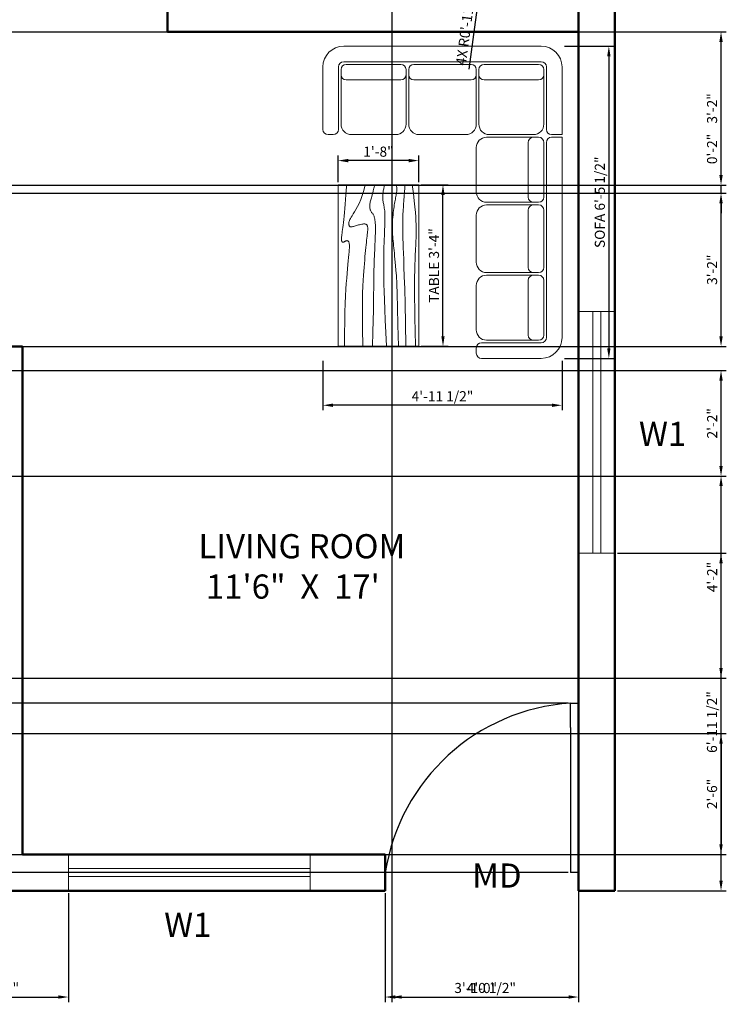
# Model space of a CAD drawing. Units: inches. Extents: x 2936 to 3364, y 2324 to 2867.
# Tile 3 of 4: x 3188 to 3364, y 2324 to 2568. Entities that reach past the tile are written whole.
import ezdxf

# ---------------------------------------------------------------- set-up
doc = ezdxf.new("R2010")
doc.units = ezdxf.units.IN
for name, color, linetype, lineweight in [('A-ANNO-DIMS', 2, 'Continuous', 18), ('A-ANNO-TEXT', 7, 'Continuous', 18), ('A-AREA-IDEN', 7, 'Continuous', 25), ('A-DOOR', 3, 'Continuous', 25), ('A-FURN', 8, 'Continuous', 18), ('A-GLAZ', 4, 'Continuous', 18), ('A-WALL', 7, 'Continuous', 50)]:
    doc.layers.add(name, color=color, linetype=linetype, lineweight=lineweight)
doc.styles.get("Standard").update_dxf_attribs({"font": 'arial.ttf'})
doc.dimstyles.new('ISO-25', dxfattribs={"dimtxt": 2.5, "dimasz": 2.5, "dimexe": 1.25, "dimexo": 0.625, "dimtad": 1, "dimdec": 0, "dimlunit": 4, "dimtxsty": 'Standard', "dimcen": 2.5, "dimadec": 0, "dimazin": 0, "dimtfac": 1, "dimtdec": 0, "dimtmove": 0, "dimatfit": 3, "dimfxl": 1, "dimarcsym": 0})

# ---------------------------------------------------------------- blocks, each defined once
blk = doc.blocks.new('Table - Rectangular Woodgrain 60 x 30 in.')
for p, q in [((0, 0), (0, -30)), ((60, 0), (0, 0)), ((60, -30), (60, 0)), ((0, -30), (60, -30))]:
    blk.add_line(p, q)
for points in [[(0, -2.4), (4.8155, -2.418), (9.0302, -2.4688), (12.709, -2.5477), (15.9167, -2.65), (18.7181, -2.7711), (21.1781, -2.9063), (23.3616, -3.0508), (25.3333, -3.2), (27.1477, -3.3495), (28.8172, -3.4958), (30.3437, -3.636), (31.7291, -3.7667), (32.9756, -3.8849), (34.0849, -3.9875), (35.059, -4.0714), (35.9, -4.1334), (36.6114, -4.1711), (37.2041, -4.1854), (37.6906, -4.1779), (38.0833, -4.15), (38.3948, -4.1034), (38.6375, -4.0396), (38.8239, -3.9602), (38.9666, -3.8667), (39.0764, -3.7608), (39.1573, -3.6448), (39.2116, -3.521), (39.2416, -3.3917), (39.2498, -3.2593), (39.2385, -3.1261), (39.21, -2.9944), (39.1666, -2.8667), (39.111, -2.7447), (39.0468, -2.6281), (38.978, -2.5163), (38.9083, -2.4083), (38.8418, -2.3035), (38.7823, -2.201), (38.7337, -2.1001), (38.7, -2), (38.6844, -1.9003), (38.6875, -1.8021), (38.7094, -1.707), (38.75, -1.6167), (38.8094, -1.5326), (38.8875, -1.4563), (38.9844, -1.3893), (39.1, -1.3333), (39.2351, -1.2896), (39.3937, -1.2583), (39.5804, -1.2396), (39.8, -1.2333), (40.057, -1.2396), (40.3562, -1.2583), (40.7023, -1.2896), (41.1, -1.3333), (41.5547, -1.3895), (42.0755, -1.4573), (42.6721, -1.5361), (43.3542, -1.625), (44.1316, -1.7233), (45.014, -1.8302), (46.0114, -1.9449), (47.1333, -2.0667), (48.3862, -2.1947), (49.7625, -2.3281), (51.2513, -2.4663), (52.8416, -2.6083), (54.5226, -2.7535), (56.2833, -2.9011), (58.1127, -3.0501), (60, -3.2)], [(0, -9.2), (6.5759, -9.0858), (11.9385, -9.0365), (16.2527, -9.0418), (19.6833, -9.0917), (22.3952, -9.1759), (24.5531, -9.2844), (26.322, -9.4069), (27.8666, -9.5333), (29.3241, -9.6553), (30.7203, -9.7719), (32.0532, -9.8837), (33.3208, -9.9917), (34.5213, -10.0965), (35.6526, -10.199), (36.7128, -10.2999), (37.7, -10.4), (38.6129, -10.4996), (39.4531, -10.5969), (40.223, -10.6895), (40.925, -10.775), (41.5613, -10.8512), (42.1344, -10.9156), (42.6465, -10.966), (43.1, -11), (43.4976, -11.0158), (43.8437, -11.0136), (44.143, -10.9942), (44.4, -10.9583), (44.6195, -10.9069), (44.8062, -10.8406), (44.9648, -10.7603), (45.1, -10.6667), (45.2155, -10.5598), (45.3114, -10.4365), (45.3871, -10.2929), (45.4416, -10.125), (45.4743, -9.929), (45.4844, -9.7011), (45.4709, -9.4371), (45.4333, -9.1333), (45.3716, -8.7883), (45.2896, -8.4104), (45.1919, -8.0107), (45.0833, -7.6), (44.9685, -7.1893), (44.8521, -6.7896), (44.7388, -6.4117), (44.6333, -6.0667), (44.54, -5.7628), (44.4614, -5.4979), (44.4001, -5.2675), (44.3583, -5.0667), (44.3384, -4.8909), (44.3427, -4.7354), (44.3736, -4.5956), (44.4333, -4.4667), (44.5236, -4.3453), (44.6427, -4.2333), (44.7884, -4.1339), (44.9583, -4.05), (45.1501, -3.9849), (45.3614, -3.9417), (45.59, -3.9234), (45.8333, -3.9333), (46.0915, -3.9749), (46.3734, -4.0531), (46.6906, -4.1736), (47.0542, -4.3417), (47.4756, -4.5629), (47.9661, -4.8427), (48.5372, -5.1866), (49.2, -5.6), (49.9676, -6.0844), (50.8594, -6.625), (51.8965, -7.2031), (53.1, -7.8), (54.491, -8.3969), (56.0906, -8.975), (57.9199, -9.5156), (60, -10)], [(0, -12.8), (5.1847, -12.9322), (9.6213, -13.0323), (13.3963, -13.1059), (16.5958, -13.1583), (19.3063, -13.1952), (21.614, -13.2219), (23.6054, -13.2439), (25.3666, -13.2667), (26.9728, -13.2947), (28.4531, -13.3281), (29.8256, -13.3663), (31.1083, -13.4083), (32.3191, -13.4535), (33.476, -13.501), (34.597, -13.5501), (35.7, -13.6), (36.7984, -13.6497), (37.8875, -13.6979), (38.9578, -13.743), (40, -13.7833), (41.0047, -13.8174), (41.9625, -13.8438), (42.864, -13.8607), (43.7, -13.8667), (44.4631, -13.8604), (45.1552, -13.8417), (45.7801, -13.8104), (46.3416, -13.7667), (46.8439, -13.7104), (47.2906, -13.6417), (47.6858, -13.5604), (48.0333, -13.4667), (48.3375, -13.3608), (48.6042, -13.2448), (48.8396, -13.121), (49.05, -12.9917), (49.2417, -12.8593), (49.4208, -12.7261), (49.5937, -12.5944), (49.7667, -12.4667), (49.9452, -12.3451), (50.1323, -12.2313), (50.3303, -12.1268), (50.5416, -12.0333), (50.7686, -11.9524), (51.0135, -11.8854), (51.2788, -11.8341), (51.5666, -11.8), (51.8785, -11.7843), (52.2116, -11.7865), (52.562, -11.8059), (52.926, -11.8417), (53.2998, -11.8931), (53.6795, -11.9594), (54.0614, -12.0397), (54.4416, -12.1333), (54.8223, -12.2401), (55.2293, -12.3625), (55.6942, -12.5037), (56.2489, -12.6667), (56.9251, -12.8547), (57.7545, -13.0708), (58.7689, -13.3182), (60, -13.6)], [(0, -18), (5.124, -17.7273), (9.6609, -17.5057), (13.6705, -17.3303), (17.2125, -17.1958), (20.3467, -17.0973), (23.1328, -17.0297), (25.6307, -16.9878), (27.9, -16.9667), (29.9928, -16.9617), (31.9302, -16.9703), (33.7254, -16.9907), (35.3917, -17.0208), (36.9423, -17.0588), (38.3906, -17.1026), (39.7499, -17.1503), (41.0333, -17.2), (42.2519, -17.2496), (43.4073, -17.2969), (44.4986, -17.3395), (45.525, -17.375), (46.4858, -17.4012), (47.3802, -17.4156), (48.2074, -17.416), (48.9667, -17.4), (49.6583, -17.3662), (50.2872, -17.3167), (50.8595, -17.2547), (51.3812, -17.1833), (51.8584, -17.1057), (52.2971, -17.025), (52.7034, -16.9443), (53.0833, -16.8667), (53.443, -16.7951), (53.789, -16.7313), (54.128, -16.6768), (54.4666, -16.6334), (54.8115, -16.6024), (55.1693, -16.5854), (55.5465, -16.5841), (55.95, -16.6), (56.3828, -16.6337), (56.8346, -16.6823), (57.2915, -16.7418), (57.7396, -16.8084), (58.165, -16.878), (58.5539, -16.9469), (58.8924, -17.0111), (59.1666, -17.0667), (59.3679, -17.1107), (59.5078, -17.1438), (59.6032, -17.1675), (59.6708, -17.1833), (59.7275, -17.193), (59.7901, -17.1979), (59.8753, -17.1998), (60, -17.2)], [(0, -22.4), (8.0098, -22.2501), (14.4094, -22.1011), (19.4168, -21.9535), (23.25, -21.8083), (26.1269, -21.6663), (28.2656, -21.5281), (29.884, -21.3947), (31.2, -21.2667), (32.3967, -21.1448), (33.5172, -21.0292), (34.5697, -20.9198), (35.5625, -20.8167), (36.5037, -20.7198), (37.4015, -20.6292), (38.2642, -20.5448), (39.1, -20.4667), (39.9164, -20.3951), (40.7187, -20.3313), (41.5117, -20.2768), (42.3, -20.2333), (43.0883, -20.2024), (43.8812, -20.1854), (44.6836, -20.1841), (45.5, -20.2), (46.3328, -20.234), (47.1747, -20.2844), (48.0163, -20.3488), (48.8479, -20.425), (49.66, -20.5106), (50.4429, -20.6031), (51.1872, -20.7004), (51.8833, -20.8), (52.5246, -20.8999), (53.1166, -20.9995), (53.6681, -21.0983), (54.1875, -21.1958), (54.6834, -21.2919), (55.1646, -21.3859), (55.6394, -21.4777), (56.1167, -21.5667), (56.6028, -21.6515), (57.0961, -21.7266), (57.5929, -21.7852), (58.0896, -21.8208), (58.5823, -21.8268), (59.0674, -21.7964), (59.5412, -21.723), (60, -21.6)], [(0, -25.2), (8.6355, -25.0504), (15.7026, -24.9031), (21.4049, -24.7606), (25.9458, -24.625), (29.529, -24.4988), (32.3578, -24.3844), (34.6359, -24.284), (36.5667, -24.2), (38.3213, -24.1341), (39.9417, -24.0854), (41.437, -24.0523), (42.8167, -24.0333), (44.0901, -24.0268), (45.2667, -24.0313), (46.3557, -24.0451), (47.3667, -24.0667), (48.309, -24.0947), (49.1928, -24.1287), (50.0284, -24.168), (50.826, -24.2125), (51.5959, -24.2617), (52.3483, -24.3151), (53.0935, -24.3725), (53.8417, -24.4334), (54.6009, -24.497), (55.3699, -24.561), (56.1454, -24.6226), (56.9239, -24.6792), (57.7021, -24.7279), (58.4764, -24.7662), (59.2435, -24.7911), (60, -24.8)], [(0, -28.8), (5.6867, -28.6681), (10.45, -28.5698), (14.407, -28.5012), (17.675, -28.4584), (20.3711, -28.4374), (22.6125, -28.4344), (24.5164, -28.4455), (26.2, -28.4667), (27.762, -28.4947), (29.2276, -28.5281), (30.6033, -28.5663), (31.8958, -28.6084), (33.1118, -28.6535), (34.2578, -28.7011), (35.3405, -28.7501), (36.3666, -28.8), (37.3443, -28.8497), (38.288, -28.8974), (39.2137, -28.9412), (40.1375, -28.9792), (41.0753, -29.0093), (42.0432, -29.0297), (43.0572, -29.0384), (44.1333, -29.0333), (45.2936, -29.0114), (46.5843, -28.9641), (48.0579, -28.8816), (49.7666, -28.7542), (51.7629, -28.5721), (54.0989, -28.3255), (56.8272, -28.0048), (60, -27.6)]]:
    blk.add_lwpolyline(points)
blk = doc.blocks.new('A$C2AFA021D')
for p, q in [((0.8, 2.3), (0.2, 2.3)), ((0.85, 2.2), (0.85, 2.25)), ((0, 2.1), (0, 0.2)), ((0.15, 0.2), (0.15, 2.1)), ((0.2, 2.15), (0.8, 2.15)), ((0.225, 2.125), (0.275, 2.125)), ((0.75, 2.125), (0.275, 2.125)), ((0.175, 1.55), (0.175, 2.075)), ((0.325, 2.075), (0.325, 1.55)), ((0.85, 1.6), (0.85, 2.025)), ((0.175, 0.875), (0.175, 1.425)), ((0.275, 1.5), (0.225, 1.5)), ((0.225, 1.475), (0.275, 1.475)), ((0.275, 1.5), (0.75, 1.5)), ((0.75, 1.475), (0.275, 1.475)), ((0.325, 1.425), (0.325, 0.875)), ((0.85, 0.925), (0.85, 1.375)), ((0.275, 0.825), (0.225, 0.825)), ((0.225, 0.8), (0.275, 0.8)), ((0.275, 0.825), (0.75, 0.825)), ((0.75, 0.8), (0.275, 0.8)), ((0.975, 0.825), (1.4, 0.825)), ((1.625, 0.825), (2.075, 0.825)), ((2.3, 0.825), (2.725, 0.825)), ((2.85, 0.2), (2.85, 0.775)), ((2.9, 0.825), (2.95, 0.825)), ((3, 0.775), (3, 0.2)), ((0.175, 0.225), (0.175, 0.75)), ((0.325, 0.75), (0.325, 0.225)), ((0.85, 0.275), (0.85, 0.7)), ((0.875, 0.275), (0.875, 0.725)), ((1.5, 0.725), (1.5, 0.275)), ((1.525, 0.275), (1.525, 0.725)), ((2.175, 0.725), (2.175, 0.275)), ((2.2, 0.275), (2.2, 0.725)), ((2.825, 0.725), (2.825, 0.275)), ((1.45, 0.325), (0.925, 0.325)), ((2.125, 0.325), (1.575, 0.325)), ((2.775, 0.325), (2.25, 0.325)), ((0.875, 0.275), (0.875, 0.225)), ((1.5, 0.225), (1.5, 0.275)), ((1.525, 0.275), (1.525, 0.225)), ((2.175, 0.225), (2.175, 0.275)), ((2.2, 0.275), (2.2, 0.225)), ((2.825, 0.225), (2.825, 0.275)), ((0.8, 0.15), (0.2, 0.15)), ((0.275, 0.175), (0.225, 0.175)), ((0.275, 0.175), (0.75, 0.175)), ((0.85, 0), (0.85, 0.1)), ((0.875, 0.1), (0.875, 0)), ((0.925, 0.175), (1.45, 0.175)), ((0.925, 0.15), (2.8, 0.15)), ((1.575, 0.175), (2.125, 0.175)), ((2.25, 0.175), (2.775, 0.175)), ((0.2, 0), (0.85, 0)), ((2.8, 0), (0.875, 0))]:
    blk.add_line(p, q)
for centre, radius, start, end in [((0.2, 2.1), 0.2, 90, 180), ((0.8, 2.25), 0.05, 0, 90), ((0.8, 2.2), 0.05, 270, 0), ((0.2, 2.1), 0.05, 90, 180), ((0.225, 2.075), 0.05, 90, 180), ((0.275, 2.075), 0.05, 0, 90), ((0.75, 2.025), 0.1, 0, 90), ((0.225, 1.55), 0.05, 180, 270), ((0.275, 1.55), 0.05, 270, 0), ((0.75, 1.6), 0.1, 270, 0), ((0.225, 1.425), 0.05, 90, 180), ((0.275, 1.425), 0.05, 0, 90), ((0.75, 1.375), 0.1, 360, 90), ((0.225, 0.875), 0.05, 180, 270), ((0.275, 0.875), 0.05, 270, 0), ((0.75, 0.925), 0.1, 270, 0), ((0.225, 0.75), 0.05, 90, 180), ((0.275, 0.75), 0.05, 0, 90), ((0.75, 0.7), 0.1, 0, 90), ((0.975, 0.725), 0.1, 90, 180), ((1.4, 0.725), 0.1, 0, 90), ((1.625, 0.725), 0.1, 90, 180), ((2.075, 0.725), 0.1, 0, 90), ((2.3, 0.725), 0.1, 90, 180), ((2.725, 0.725), 0.1, 0, 90), ((2.9, 0.775), 0.05, 90, 180), ((2.95, 0.775), 0.05, 0, 90), ((0.925, 0.275), 0.05, 90, 180), ((1.45, 0.275), 0.05, 360, 90), ((1.575, 0.275), 0.05, 90, 180), ((2.125, 0.275), 0.05, 360, 90), ((2.25, 0.275), 0.05, 90, 180), ((2.775, 0.275), 0.05, 360, 90), ((0.2, 0.2), 0.2, 180, 270), ((0.2, 0.2), 0.05, 180, 270), ((0.225, 0.225), 0.05, 180, 270), ((0.275, 0.225), 0.05, 270, 0), ((0.75, 0.275), 0.1, 270, 0), ((0.925, 0.225), 0.05, 180, 270), ((1.45, 0.225), 0.05, 270, 0), ((1.575, 0.225), 0.05, 180, 270), ((2.125, 0.225), 0.05, 270, 0), ((2.25, 0.225), 0.05, 180, 270), ((2.775, 0.225), 0.05, 270, 0), ((2.8, 0.2), 0.2, 270, 0), ((2.8, 0.2), 0.05, 270, 0), ((0.8, 0.1), 0.05, 0, 90), ((0.925, 0.1), 0.05, 90, 180)]:
    blk.add_arc(centre, radius, start, end)
blk = doc.blocks.new('WIN-W1-60IN')
for p, q in [((3.5, 60), (3.5, 0)), ((5.5, 60), (5.5, 0))]:
    blk.add_line(p, q)
blk.add_lwpolyline([(0, 0), (9, 0), (9, 60), (0, 60)], close=True)
blk = doc.blocks.new('*D29')
at = {"layer": 'A-ANNO-DIMS', "color": 0, "lineweight": -2, "transparency": 16777216}
for p, q in [((3288.13, 2527.16), (3294.76, 2527.16)), ((3293.51, 2489.63), (3293.51, 2524.66)), ((3288.13, 2487.13), (3294.76, 2487.13))]:
    blk.add_line(p, q, dxfattribs=at)
at = {"layer": 'A-ANNO-DIMS', "color": 0, "transparency": 16777216}
for points in [[(3293.09, 2524.66), (3293.92, 2524.66), (3293.51, 2527.16)], [(3293.09, 2489.63), (3293.92, 2489.63), (3293.51, 2487.13)]]:
    blk.add_solid(points, dxfattribs=at)
at = {"layer": 'Defpoints', "color": 0, "transparency": 16777216}
for p in [(3287.5, 2527.16), (3293.51, 2527.16), (3287.5, 2487.13)]:
    blk.add_point(p, dxfattribs=at)
at = {"layer": 'A-ANNO-DIMS', "color": 0, "transparency": 16777216, "insert": (3291.6, 2507.15), "char_height": 2.5, "attachment_point": 5, "rotation": 90}
blk.add_mtext('TABLE 3\'-4"', dxfattribs=at)
blk = doc.blocks.new('*D30')
at = {"layer": 'A-ANNO-DIMS', "color": 0, "lineweight": -2, "transparency": 16777216}
for p, q in [((3267.48, 2527.79), (3267.48, 2534.42)), ((3287.5, 2527.79), (3287.5, 2534.42)), ((3285, 2533.17), (3269.98, 2533.17))]:
    blk.add_line(p, q, dxfattribs=at)
at = {"layer": 'A-ANNO-DIMS', "color": 0, "transparency": 16777216}
for points in [[(3269.98, 2533.59), (3269.98, 2532.75), (3267.48, 2533.17)], [(3285, 2533.59), (3285, 2532.75), (3287.5, 2533.17)]]:
    blk.add_solid(points, dxfattribs=at)
at = {"layer": 'Defpoints', "color": 0, "transparency": 16777216}
for p in [(3267.48, 2533.17), (3267.48, 2527.16), (3287.5, 2527.16)]:
    blk.add_point(p, dxfattribs=at)
at = {"layer": 'A-ANNO-DIMS', "color": 0, "transparency": 16777216, "insert": (3277.49, 2535.07), "char_height": 2.5, "attachment_point": 5}
blk.add_mtext('1\'-8"', dxfattribs=at)
blk = doc.blocks.new('*D31')
at = {"layer": 'A-ANNO-DIMS', "color": 0, "lineweight": -2, "transparency": 16777216}
for p, q in [((3323.69, 2561.55), (3335.93, 2561.55)), ((3334.68, 2559.05), (3334.68, 2486.62)), ((3323.69, 2484.12), (3335.93, 2484.12))]:
    blk.add_line(p, q, dxfattribs=at)
at = {"layer": 'A-ANNO-DIMS', "color": 0, "transparency": 16777216}
for points in [[(3334.26, 2559.05), (3335.09, 2559.05), (3334.68, 2561.55)], [(3334.26, 2486.62), (3335.09, 2486.62), (3334.68, 2484.12)]]:
    blk.add_solid(points, dxfattribs=at)
at = {"layer": 'Defpoints', "color": 0, "transparency": 16777216}
for p in [(3323.06, 2561.55), (3323.06, 2484.12), (3334.68, 2484.12)]:
    blk.add_point(p, dxfattribs=at)
at = {"layer": 'A-ANNO-DIMS', "color": 0, "transparency": 16777216, "insert": (3332.76, 2522.84), "char_height": 2.5, "attachment_point": 5, "rotation": 90}
blk.add_mtext('SOFA 6\'-5 1/2"', dxfattribs=at)
blk = doc.blocks.new('*D32')
at = {"layer": 'A-ANNO-DIMS', "color": 0, "lineweight": -2, "transparency": 16777216}
for p, q in [((3263.7, 2483.49), (3263.7, 2471.25)), ((3323.06, 2483.49), (3323.06, 2471.25)), ((3320.56, 2472.5), (3266.2, 2472.5))]:
    blk.add_line(p, q, dxfattribs=at)
at = {"layer": 'A-ANNO-DIMS', "color": 0, "transparency": 16777216}
for points in [[(3266.2, 2472.92), (3266.2, 2472.09), (3263.7, 2472.5)], [(3320.56, 2472.92), (3320.56, 2472.09), (3323.06, 2472.5)]]:
    blk.add_solid(points, dxfattribs=at)
at = {"layer": 'Defpoints', "color": 0, "transparency": 16777216}
for p in [(3263.7, 2484.12), (3323.06, 2484.12), (3263.7, 2472.5)]:
    blk.add_point(p, dxfattribs=at)
at = {"layer": 'A-ANNO-DIMS', "color": 0, "transparency": 16777216, "insert": (3293.38, 2474.42), "char_height": 2.5, "attachment_point": 5, "rotation": 360}
blk.add_mtext('4\'-11 1/2"', dxfattribs=at)
blk = doc.blocks.new('*D37')
at = {"layer": 'A-ANNO-DIMS', "color": 0, "lineweight": -2, "transparency": 16777216}
for p, q in [((3279.17, 2351.49), (3279.17, 2324.51)), ((3327.17, 2351.49), (3327.17, 2324.51)), ((3281.67, 2325.76), (3324.67, 2325.76))]:
    blk.add_line(p, q, dxfattribs=at)
at = {"layer": 'A-ANNO-DIMS', "color": 0, "transparency": 16777216}
for points in [[(3281.67, 2326.18), (3281.67, 2325.35), (3279.17, 2325.76)], [(3324.67, 2326.18), (3324.67, 2325.35), (3327.17, 2325.76)]]:
    blk.add_solid(points, dxfattribs=at)
at = {"layer": 'Defpoints', "color": 0, "transparency": 16777216}
for p in [(3279.17, 2352.11), (3327.17, 2352.11), (3327.17, 2325.76)]:
    blk.add_point(p, dxfattribs=at)
at = {"layer": 'A-ANNO-DIMS', "color": 0, "transparency": 16777216, "insert": (3303.17, 2327.67), "char_height": 2.5, "attachment_point": 5}
blk.add_mtext('4\'-0"', dxfattribs=at)
blk = doc.blocks.new('*D42')
at = {"layer": 'A-ANNO-DIMS', "color": 0, "lineweight": -2, "transparency": 16777216}
for p, q in [((3336.79, 2435.79), (3363.77, 2435.79)), ((3362.52, 2354.61), (3362.52, 2433.29)), ((3336.79, 2352.11), (3363.77, 2352.11))]:
    blk.add_line(p, q, dxfattribs=at)
at = {"layer": 'A-ANNO-DIMS', "color": 0, "transparency": 16777216}
for points in [[(3362.1, 2433.29), (3362.94, 2433.29), (3362.52, 2435.79)], [(3362.1, 2354.61), (3362.94, 2354.61), (3362.52, 2352.11)]]:
    blk.add_solid(points, dxfattribs=at)
at = {"layer": 'Defpoints', "color": 0, "transparency": 16777216}
for p in [(3336.17, 2435.79), (3362.52, 2435.79), (3336.17, 2352.11)]:
    blk.add_point(p, dxfattribs=at)
at = {"layer": 'A-ANNO-DIMS', "color": 0, "transparency": 16777216, "insert": (3360.6, 2393.95), "char_height": 2.5, "attachment_point": 5, "rotation": 90}
blk.add_mtext('6\'-11 1/2"', dxfattribs=at)
blk = doc.blocks.new('*D44')
at = {"layer": 'A-ANNO-DIMS', "color": 0, "lineweight": -2, "transparency": 16777216}
for p, q in [((3280.77, 2822.49), (3280.77, 2324.51)), ((3327.17, 2822.49), (3327.17, 2324.51)), ((3283.27, 2325.76), (3324.67, 2325.76))]:
    blk.add_line(p, q, dxfattribs=at)
at = {"layer": 'A-ANNO-DIMS', "color": 0, "transparency": 16777216}
for points in [[(3283.27, 2326.18), (3283.27, 2325.35), (3280.77, 2325.76)], [(3324.67, 2326.18), (3324.67, 2325.35), (3327.17, 2325.76)]]:
    blk.add_solid(points, dxfattribs=at)
at = {"layer": 'Defpoints', "color": 0, "transparency": 16777216}
for p in [(3280.77, 2823.11), (3327.17, 2823.11), (3327.17, 2325.76)]:
    blk.add_point(p, dxfattribs=at)
at = {"layer": 'A-ANNO-DIMS', "color": 0, "transparency": 16777216, "insert": (3303.97, 2327.68), "char_height": 2.5, "attachment_point": 5}
blk.add_mtext('3\'-10 1/2"', dxfattribs=at)
blk = doc.blocks.new('*D46')
at = {"layer": 'A-ANNO-DIMS', "color": 0, "lineweight": -2, "transparency": 16777216}
for p, q in [((3166.62, 2351.49), (3166.62, 2324.51)), ((3200.55, 2351.49), (3200.55, 2324.51)), ((3169.12, 2325.76), (3198.05, 2325.76))]:
    blk.add_line(p, q, dxfattribs=at)
at = {"layer": 'A-ANNO-DIMS', "color": 0, "transparency": 16777216}
for points in [[(3169.12, 2326.18), (3169.12, 2325.35), (3166.62, 2325.76)], [(3198.05, 2326.18), (3198.05, 2325.35), (3200.55, 2325.76)]]:
    blk.add_solid(points, dxfattribs=at)
at = {"layer": 'Defpoints', "color": 0, "transparency": 16777216}
for p in [(3166.62, 2352.11), (3200.55, 2352.11), (3200.55, 2325.76)]:
    blk.add_point(p, dxfattribs=at)
at = {"layer": 'A-ANNO-DIMS', "color": 0, "transparency": 16777216, "insert": (3183.58, 2327.67), "char_height": 2.5, "attachment_point": 5}
blk.add_mtext('2\'-10"', dxfattribs=at)
blk = doc.blocks.new('*D50')
at = {"layer": 'A-ANNO-DIMS', "color": 0, "lineweight": -2, "transparency": 16777216}
for p, q in [((3121.79, 2525.11), (3363.77, 2525.11)), ((3362.52, 2489.61), (3362.52, 2522.61)), ((3121.79, 2487.11), (3363.77, 2487.11))]:
    blk.add_line(p, q, dxfattribs=at)
at = {"layer": 'A-ANNO-DIMS', "color": 0, "transparency": 16777216}
for points in [[(3362.1, 2522.61), (3362.94, 2522.61), (3362.52, 2525.11)], [(3362.1, 2489.61), (3362.94, 2489.61), (3362.52, 2487.11)]]:
    blk.add_solid(points, dxfattribs=at)
at = {"layer": 'Defpoints', "color": 0, "transparency": 16777216}
for p in [(3121.17, 2525.11), (3362.52, 2525.11), (3121.17, 2487.11)]:
    blk.add_point(p, dxfattribs=at)
at = {"layer": 'A-ANNO-DIMS', "color": 0, "transparency": 16777216, "insert": (3360.62, 2506.11), "char_height": 2.5, "attachment_point": 5, "rotation": 90}
blk.add_mtext('3\'-2"', dxfattribs=at)
blk = doc.blocks.new('*D54')
at = {"layer": 'A-ANNO-DIMS', "color": 0, "lineweight": -2, "transparency": 16777216}
for p, q in [((3087.79, 2454.95), (3363.77, 2454.95)), ((3362.52, 2407.37), (3362.52, 2452.45)), ((3087.79, 2404.87), (3363.77, 2404.87))]:
    blk.add_line(p, q, dxfattribs=at)
at = {"layer": 'A-ANNO-DIMS', "color": 0, "transparency": 16777216}
for points in [[(3362.1, 2452.45), (3362.94, 2452.45), (3362.52, 2454.95)], [(3362.1, 2407.37), (3362.94, 2407.37), (3362.52, 2404.87)]]:
    blk.add_solid(points, dxfattribs=at)
at = {"layer": 'Defpoints', "color": 0, "transparency": 16777216}
for p in [(3087.17, 2454.95), (3362.52, 2454.95), (3087.17, 2404.87)]:
    blk.add_point(p, dxfattribs=at)
at = {"layer": 'A-ANNO-DIMS', "color": 0, "transparency": 16777216, "insert": (3360.64, 2429.91), "char_height": 2.5, "attachment_point": 5, "rotation": 90}
blk.add_mtext('4\'-2"', dxfattribs=at)
blk = doc.blocks.new('*D55')
at = {"layer": 'A-ANNO-DIMS', "color": 0, "lineweight": -2, "transparency": 16777216}
for p, q in [((3087.79, 2481.11), (3363.77, 2481.11)), ((3362.52, 2457.45), (3362.52, 2478.61)), ((3087.79, 2454.95), (3363.77, 2454.95))]:
    blk.add_line(p, q, dxfattribs=at)
at = {"layer": 'A-ANNO-DIMS', "color": 0, "transparency": 16777216}
for points in [[(3362.1, 2478.61), (3362.94, 2478.61), (3362.52, 2481.11)], [(3362.1, 2457.45), (3362.94, 2457.45), (3362.52, 2454.95)]]:
    blk.add_solid(points, dxfattribs=at)
at = {"layer": 'Defpoints', "color": 0, "transparency": 16777216}
for p in [(3087.17, 2481.11), (3362.52, 2481.11), (3087.17, 2454.95)]:
    blk.add_point(p, dxfattribs=at)
at = {"layer": 'A-ANNO-DIMS', "color": 0, "transparency": 16777216, "insert": (3360.64, 2468.03), "char_height": 2.5, "attachment_point": 5, "rotation": 90}
blk.add_mtext('2\'-2"', dxfattribs=at)
blk = doc.blocks.new('*D56')
at = {"layer": 'A-ANNO-DIMS', "color": 0, "lineweight": -2, "transparency": 16777216}
for p, q in [((3081.79, 2391.11), (3363.77, 2391.11)), ((3362.52, 2388.61), (3362.52, 2363.61)), ((3081.79, 2361.11), (3363.77, 2361.11))]:
    blk.add_line(p, q, dxfattribs=at)
at = {"layer": 'A-ANNO-DIMS', "color": 0, "transparency": 16777216}
for points in [[(3362.1, 2388.61), (3362.94, 2388.61), (3362.52, 2391.11)], [(3362.1, 2363.61), (3362.94, 2363.61), (3362.52, 2361.11)]]:
    blk.add_solid(points, dxfattribs=at)
at = {"layer": 'Defpoints', "color": 0, "transparency": 16777216}
for p in [(3081.17, 2391.11), (3081.17, 2361.11), (3362.52, 2361.11)]:
    blk.add_point(p, dxfattribs=at)
at = {"layer": 'A-ANNO-DIMS', "color": 0, "transparency": 16777216, "insert": (3360.62, 2376.11), "char_height": 2.5, "attachment_point": 5, "rotation": 90}
blk.add_mtext('2\'-6"', dxfattribs=at)
blk = doc.blocks.new('*D59')
at = {"layer": 'A-ANNO-DIMS', "color": 0, "lineweight": -2, "transparency": 16777216}
for p, q in [((3111.79, 2565.11), (3363.77, 2565.11)), ((3362.52, 2529.61), (3362.52, 2562.61)), ((3111.79, 2527.11), (3363.77, 2527.11))]:
    blk.add_line(p, q, dxfattribs=at)
at = {"layer": 'A-ANNO-DIMS', "color": 0, "transparency": 16777216}
for points in [[(3362.1, 2562.61), (3362.94, 2562.61), (3362.52, 2565.11)], [(3362.1, 2529.61), (3362.94, 2529.61), (3362.52, 2527.11)]]:
    blk.add_solid(points, dxfattribs=at)
at = {"layer": 'Defpoints', "color": 0, "transparency": 16777216}
for p in [(3111.17, 2565.11), (3362.52, 2565.11), (3111.17, 2527.11)]:
    blk.add_point(p, dxfattribs=at)
at = {"layer": 'A-ANNO-DIMS', "color": 0, "transparency": 16777216, "insert": (3360.62, 2546.11), "char_height": 2.5, "attachment_point": 5, "rotation": 90}
blk.add_mtext('3\'-2"', dxfattribs=at)
blk = doc.blocks.new('*D60')
at = {"layer": 'A-ANNO-DIMS', "color": 0, "lineweight": -2, "transparency": 16777216}
for p, q in [((3362.52, 2529.61), (3362.52, 2540.01)), ((3111.79, 2527.11), (3363.77, 2527.11)), ((3362.52, 2525.11), (3362.52, 2527.11)), ((3111.79, 2525.11), (3363.77, 2525.11)), ((3362.52, 2522.61), (3362.52, 2520.11))]:
    blk.add_line(p, q, dxfattribs=at)
at = {"layer": 'A-ANNO-DIMS', "color": 0, "transparency": 16777216}
for points in [[(3362.1, 2529.61), (3362.94, 2529.61), (3362.52, 2527.11)], [(3362.1, 2522.61), (3362.94, 2522.61), (3362.52, 2525.11)]]:
    blk.add_solid(points, dxfattribs=at)
at = {"layer": 'Defpoints', "color": 0, "transparency": 16777216}
for p in [(3111.17, 2527.11), (3362.52, 2527.11), (3111.17, 2525.11)]:
    blk.add_point(p, dxfattribs=at)
at = {"layer": 'A-ANNO-DIMS', "color": 0, "transparency": 16777216, "insert": (3360.62, 2536.06), "char_height": 2.5, "attachment_point": 5, "rotation": 90}
blk.add_mtext('0\'-2"', dxfattribs=at)
blk = doc.blocks.new('*D64')
at = {"layer": 'A-ANNO-DIMS', "color": 0, "lineweight": -2, "transparency": 16777216}
for p, q in [((3324.54, 2398.61), (2948.57, 2398.61)), ((2949.82, 2359.11), (2949.82, 2396.11)), ((3324.54, 2356.61), (2948.57, 2356.61))]:
    blk.add_line(p, q, dxfattribs=at)
at = {"layer": 'A-ANNO-DIMS', "color": 0, "transparency": 16777216}
for points in [[(2949.4, 2396.11), (2950.24, 2396.11), (2949.82, 2398.61)], [(2949.4, 2359.11), (2950.24, 2359.11), (2949.82, 2356.61)]]:
    blk.add_solid(points, dxfattribs=at)
at = {"layer": 'Defpoints', "color": 0, "transparency": 16777216}
for p in [(2949.82, 2398.61), (3325.17, 2398.61), (3325.17, 2356.61)]:
    blk.add_point(p, dxfattribs=at)
at = {"layer": 'A-ANNO-DIMS', "color": 0, "transparency": 16777216, "insert": (2947.92, 2377.61), "char_height": 2.5, "attachment_point": 5, "rotation": 90}
blk.add_mtext('3\'-6"', dxfattribs=at)
blk = doc.blocks.new('*D66')
at = {"layer": 'A-ANNO-DIMS', "color": 0, "lineweight": -2, "transparency": 16777216}
for p, q in [((3305.35, 2595.31), (3303.84, 2584.09)), ((3300.04, 2555.81), (3303.51, 2581.61))]:
    blk.add_line(p, q, dxfattribs=at)
at = {"layer": 'A-ANNO-DIMS', "color": 0, "transparency": 16777216}
blk.add_solid([(3303.1, 2581.66), (3303.92, 2581.55), (3303.84, 2584.09)], dxfattribs=at)
at = {"layer": 'Defpoints', "color": 0, "transparency": 16777216}
for p in [(3305.35, 2595.31), (3303.84, 2584.09)]:
    blk.add_point(p, dxfattribs=at)
at = {"layer": 'A-ANNO-DIMS', "color": 0, "transparency": 16777216, "insert": (3299.71, 2567.73), "char_height": 2.5, "attachment_point": 5, "rotation": 82.3437}
blk.add_mtext('4X R0\'-11 1/2"', dxfattribs=at)

msp = doc.modelspace()

# ---------------------------------------------------------------- linework, layer by layer
at = {"layer": 'A-DOOR'}
for p, q in [((3325.17, 2392.61), (3325.17, 2398.61)), ((3325.17, 2398.61), (3327.17, 2398.61)), ((3325.17, 2392.61), (3325.17, 2356.61)), ((3327.17, 2356.61), (3327.17, 2392.61)), ((3279.17, 2356.61), (3279.17, 2361.11)), ((3327.17, 2356.61), (3327.17, 2358.61)), ((3327.17, 2356.61), (3325.17, 2356.61))]:
    msp.add_line(p, q, dxfattribs=at)
msp.add_arc((3328.38, 2348.91), 49.81, 93.6972, 171.0976, dxfattribs=at)
at = {"layer": 'A-WALL'}
for p, q in [((3225.17, 2565.11), (3225.17, 2643.11)), ((3327.17, 2487.11), (3327.17, 2643.11)), ((3327.17, 2565.11), (3225.17, 2565.11)), ((3183.17, 2487.11), (3189.17, 2487.11)), ((3189.17, 2487.11), (3189.17, 2361.11)), ((3327.17, 2361.11), (3327.17, 2487.11)), ((3189.17, 2361.11), (3279.17, 2361.11)), ((3279.17, 2361.11), (3279.17, 2352.11)), ((3327.17, 2361.11), (3327.17, 2352.11)), ((3327.17, 2352.11), (3336.17, 2352.11))]:
    msp.add_line(p, q, dxfattribs=at)
msp.add_lwpolyline([(3336.17, 2352.11), (3336.17, 2832.11), (2976.17, 2832.11), (2976.17, 2352.11), (3279.17, 2352.11)], dxfattribs=at)

# ---------------------------------------------------------------- block references
at = {"layer": 'A-FURN'}
for name, p, xscale, yscale, zscale, rotation in [('A$C2AFA021D', (3323.06, 2561.55), -25.81059154860956, 25.81059154860955, 25.81059154860955, 89.99998967457302), ('Table - Rectangular Woodgrain 60 x 30 in.', (3267.48, 2487.13), 0.667224614481091, 0.667224614481091, 0.667224614481091, 90)]:
    msp.add_blockref(name, p, dxfattribs=dict(at, xscale=xscale, yscale=yscale, zscale=zscale, rotation=rotation))
at = {"layer": 'A-GLAZ'}
msp.add_blockref('WIN-W1-60IN', (3327.17, 2435.79), dxfattribs=at)
at = {"layer": 'A-GLAZ', "rotation": 90.00000000000078}
msp.add_blockref('WIN-W1-60IN', (3260.55, 2352.11), dxfattribs=at)

# ---------------------------------------------------------------- texts
at = {"layer": 'A-ANNO-TEXT', "char_height": 6, "attachment_point": 1}
for s, width, heights, insert in [('W1', 56.3393, [0], (3342.15, 2468.4)), ('MD', 67.7516, [9.32], (3300.74, 2358.88)), ('W1', 56.3393, [0], (3224.31, 2346.68))]:
    msp.add_mtext_dynamic_manual_height_columns(s, width=width, gutter_width=12.5, heights=heights, dxfattribs=dict(at, insert=insert))
at = {"layer": 'A-AREA-IDEN', "insert": (3232.82, 2440.54), "char_height": 6, "attachment_point": 1}
msp.add_mtext_dynamic_manual_height_columns('LIVING ROOM\\P 11\'6"  X  17\'', width=56.3393, gutter_width=12.5, heights=[0], dxfattribs=at)

# ---------------------------------------------------------------- dimensions: what is measured, and where the dimension line sits
at = {"layer": 'A-ANNO-DIMS'}
for base, p1, p2, picture, middle in [((3327.17, 2325.76), (3280.77, 2823.11), (3327.17, 2823.11), '*D44', (3303.97, 2327.68)), ((3200.55, 2325.76), (3166.62, 2352.11), (3200.55, 2352.11), '*D46', (3183.58, 2327.67)), ((3327.17, 2325.76), (3279.17, 2352.11), (3327.17, 2352.11), '*D37', (3303.17, 2327.67))]:
    dim = msp.add_linear_dim(base=base, p1=p1, p2=p2, dimstyle='ISO-25', override={"dimdec": 1, "dimlfac": 1, "dimrnd": 0, "dimzin": 1, "dimdsep": 46, "dimlunit": 4, "dimfrac": 2}, dxfattribs=at)
    dim.commit()
    dim.dimension.update_dxf_attribs({"geometry": picture, "text_midpoint": middle})
dim = msp.add_radius_dim(center=(3305.35, 2595.31), mpoint=(3303.84, 2584.09), text='4X <>', dimstyle='ISO-25', override={"dimdec": 1, "dimlfac": 1, "dimrnd": 0, "dimzin": 1, "dimdsep": 46, "dimlunit": 4, "dimfrac": 2}, dxfattribs=at)
dim.commit()
dim.dimension.update_dxf_attribs({"geometry": '*D66', "text_midpoint": (3299.71, 2567.73)})
for base, p1, p2, angle, picture, middle in [((3362.52, 2565.11), (3111.17, 2527.11), (3111.17, 2565.11), 90, '*D59', (3360.62, 2546.11)), ((3362.52, 2527.11), (3111.17, 2525.11), (3111.17, 2527.11), 90, '*D60', (3360.62, 2536.06)), ((3267.48, 2533.17), (3287.5, 2527.16), (3267.48, 2527.16), 180, '*D30', (3277.49, 2535.07)), ((3362.52, 2525.11), (3121.17, 2487.11), (3121.17, 2525.11), 90, '*D50', (3360.62, 2506.11)), ((3263.7, 2472.5), (3323.06, 2484.12), (3263.7, 2484.12), 180, '*D32', (3293.38, 2474.42)), ((3362.52, 2481.11), (3087.17, 2454.95), (3087.17, 2481.11), 90, '*D55', (3360.64, 2468.03)), ((3362.52, 2454.95), (3087.17, 2404.87), (3087.17, 2454.95), 90, '*D54', (3360.64, 2429.91)), ((3362.52, 2435.79), (3336.17, 2352.11), (3336.17, 2435.79), 90, '*D42', (3360.6, 2393.95)), ((2949.82, 2398.61), (3325.17, 2356.61), (3325.17, 2398.61), 90, '*D64', (2947.92, 2377.61)), ((3362.52, 2361.11), (3081.17, 2391.11), (3081.17, 2361.11), 90, '*D56', (3360.62, 2376.11))]:
    dim = msp.add_linear_dim(base=base, p1=p1, p2=p2, angle=angle, dimstyle='ISO-25', override={"dimdec": 1, "dimlfac": 1, "dimrnd": 0, "dimzin": 1, "dimdsep": 46, "dimlunit": 4, "dimfrac": 2}, dxfattribs=at)
    dim.commit()
    dim.dimension.update_dxf_attribs({"geometry": picture, "text_midpoint": middle})
for base, p1, p2, angle, text, picture, middle in [((3334.68, 2484.12), (3323.06, 2561.55), (3323.06, 2484.12), 270, 'SOFA <>', '*D31', (3332.76, 2522.84)), ((3293.51, 2527.16), (3287.5, 2487.13), (3287.5, 2527.16), 90, 'TABLE <>', '*D29', (3291.6, 2507.15))]:
    dim = msp.add_linear_dim(base=base, p1=p1, p2=p2, angle=angle, text=text, dimstyle='ISO-25', override={"dimdec": 1, "dimlfac": 1, "dimrnd": 0, "dimzin": 1, "dimdsep": 46, "dimlunit": 4, "dimfrac": 2}, dxfattribs=at)
    dim.commit()
    dim.dimension.update_dxf_attribs({"geometry": picture, "text_midpoint": middle})

doc.saveas('drawing.dxf')
